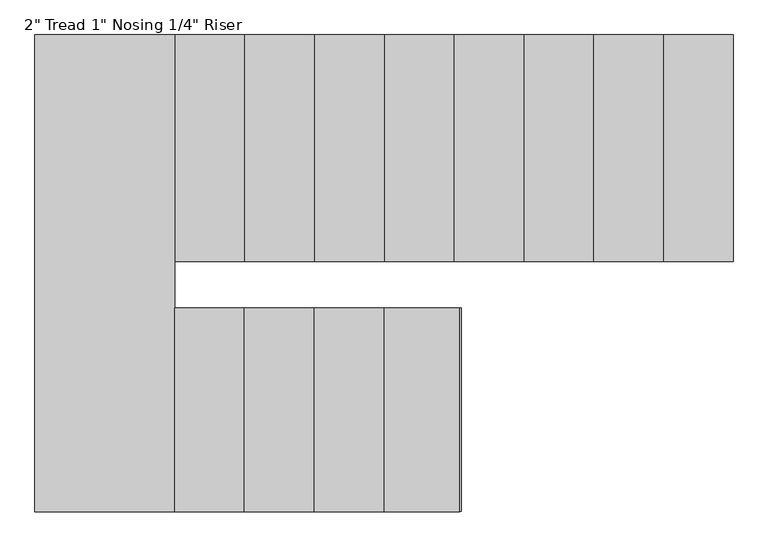
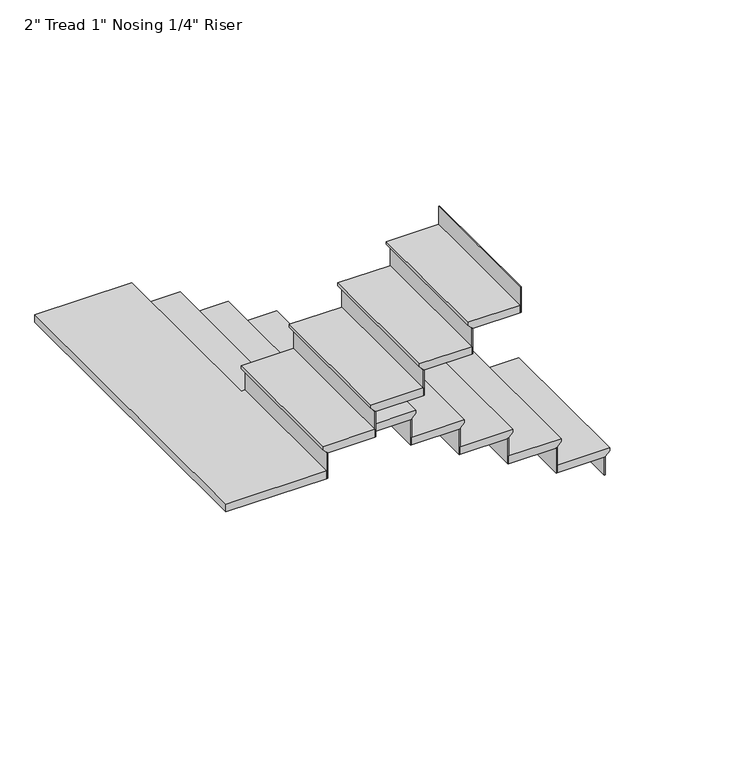
"""IFC4 building model written with IfcOpenShell, lengths in millimetres: stair flight geometry."""

from ifc_helpers import new_model, si_unit, origin, place, context, project, spatial, faceted_brep, source, transform, mapped, element, save


def stair_flight_d10e185a(model_context):
    return source(origin(), model_context, "Body", "Brep", [
        faceted_brep([(-569.5630704, 657.3457979, 3198.2833333), (-569.5630704, 657.3457979, 3217.3333333), (-569.5630704, -333.2542021, 3217.3333333), (-569.5630704, -333.2542021, 3198.2833333), (-594.9630704, 657.3457979, 3172.8833333), (-594.9630704, -333.2542021, 3172.8833333), (-899.7630704, 657.3457979, 3217.3333333), (-899.7630704, -333.2542021, 3217.3333333), (-594.9630704, -333.2542021, 3166.5333333), (-899.7630704, -333.2542021, 3166.5333333), (-899.7630704, 657.3457979, 3166.5333333), (-594.9630704, 657.3457979, 3166.5333333)], [[[0, 1, 2, 3]], [[4, 0, 3, 5]], [[2, 1, 6, 7]], [[8, 9, 10, 11]], [[2, 7, 9, 8, 5, 3]], [[8, 11, 4, 5]], [[6, 1, 0, 4, 11, 10]], [[7, 6, 10, 9]]]),
        faceted_brep([(-594.9630704, 657.3457979, 3166.5333333), (-594.9630704, 657.3457979, 3048.0), (-601.3130704, 657.3457979, 3048.0), (-601.3130704, 657.3457979, 3166.5333333), (-594.9630704, -333.2542021, 3166.5333333), (-601.3130704, -333.2542021, 3166.5333333), (-601.3130704, -333.2542021, 3048.0), (-594.9630704, -333.2542021, 3048.0)], [[[0, 1, 2, 3]], [[4, 5, 6, 7]], [[1, 0, 4, 7]], [[2, 1, 7, 6]], [[3, 2, 6, 5]], [[0, 3, 5, 4]]]),
        faceted_brep([(-899.7630704, 657.3457979, 3335.8666667), (-899.7630704, 657.3457979, 3166.5333333), (-906.1130704, 657.3457979, 3166.5333333), (-906.1130704, 657.3457979, 3335.8666667), (-899.7630704, -333.2542021, 3335.8666667), (-906.1130704, -333.2542021, 3335.8666667), (-906.1130704, -333.2542021, 3166.5333333), (-899.7630704, -333.2542021, 3166.5333333)], [[[0, 1, 2, 3]], [[4, 5, 6, 7]], [[1, 0, 4, 7]], [[2, 1, 7, 6]], [[3, 2, 6, 5]], [[0, 3, 5, 4]]]),
        faceted_brep([(-874.3630704, -333.2542021, 3386.6666667), (-874.3630704, 657.3457979, 3386.6666667), (-1204.5630704, 657.3457979, 3386.6666667), (-1204.5630704, -333.2542021, 3386.6666667), (-899.7630704, -333.2542021, 3335.8666667), (-1204.5630704, -333.2542021, 3335.8666667), (-1204.5630704, 657.3457979, 3335.8666667), (-899.7630704, 657.3457979, 3335.8666667), (-899.7630704, -333.2542021, 3342.2166667), (-874.3630704, -333.2542021, 3367.6166667), (-899.7630704, 657.3457979, 3342.2166667), (-874.3630704, 657.3457979, 3367.6166667)], [[[0, 1, 2, 3]], [[4, 5, 6, 7]], [[0, 3, 5, 4, 8, 9]], [[4, 7, 10, 8]], [[2, 1, 11, 10, 7, 6]], [[3, 2, 6, 5]], [[11, 1, 0, 9]], [[10, 11, 9, 8]]]),
        faceted_brep([(-1204.5630704, 657.3457979, 3505.2), (-1204.5630704, 657.3457979, 3335.8666667), (-1210.9130704, 657.3457979, 3335.8666667), (-1210.9130704, 657.3457979, 3505.2), (-1204.5630704, -333.2542021, 3505.2), (-1210.9130704, -333.2542021, 3505.2), (-1210.9130704, -333.2542021, 3335.8666667), (-1204.5630704, -333.2542021, 3335.8666667)], [[[0, 1, 2, 3]], [[4, 5, 6, 7]], [[1, 0, 4, 7]], [[2, 1, 7, 6]], [[3, 2, 6, 5]], [[0, 3, 5, 4]]]),
        faceted_brep([(-1179.1630704, -333.2542021, 3556.0), (-1179.1630704, 657.3457979, 3556.0), (-1509.3630704, 657.3457979, 3556.0), (-1509.3630704, -333.2542021, 3556.0), (-1204.5630704, -333.2542021, 3505.2), (-1509.3630704, -333.2542021, 3505.2), (-1509.3630704, 657.3457979, 3505.2), (-1204.5630704, 657.3457979, 3505.2), (-1204.5630704, -333.2542021, 3511.55), (-1179.1630704, -333.2542021, 3536.95), (-1204.5630704, 657.3457979, 3511.55), (-1179.1630704, 657.3457979, 3536.95)], [[[0, 1, 2, 3]], [[4, 5, 6, 7]], [[0, 3, 5, 4, 8, 9]], [[4, 7, 10, 8]], [[2, 1, 11, 10, 7, 6]], [[3, 2, 6, 5]], [[11, 1, 0, 9]], [[10, 11, 9, 8]]]),
        faceted_brep([(-1509.3630704, 657.3457979, 3674.5333333), (-1509.3630704, 657.3457979, 3505.2), (-1515.7130704, 657.3457979, 3505.2), (-1515.7130704, 657.3457979, 3674.5333333), (-1509.3630704, -333.2542021, 3674.5333333), (-1515.7130704, -333.2542021, 3674.5333333), (-1515.7130704, -333.2542021, 3505.2), (-1509.3630704, -333.2542021, 3505.2)], [[[0, 1, 2, 3]], [[4, 5, 6, 7]], [[1, 0, 4, 7]], [[2, 1, 7, 6]], [[3, 2, 6, 5]], [[0, 3, 5, 4]]]),
        faceted_brep([(-1483.9630704, -333.2542021, 3725.3333333), (-1483.9630704, 657.3457979, 3725.3333333), (-1814.1630704, 657.3457979, 3725.3333333), (-1814.1630704, -333.2542021, 3725.3333333), (-1509.3630704, -333.2542021, 3674.5333333), (-1814.1630704, -333.2542021, 3674.5333333), (-1814.1630704, 657.3457979, 3674.5333333), (-1509.3630704, 657.3457979, 3674.5333333), (-1509.3630704, -333.2542021, 3680.8833333), (-1483.9630704, -333.2542021, 3706.2833333), (-1509.3630704, 657.3457979, 3680.8833333), (-1483.9630704, 657.3457979, 3706.2833333)], [[[0, 1, 2, 3]], [[4, 5, 6, 7]], [[0, 3, 5, 4, 8, 9]], [[4, 7, 10, 8]], [[2, 1, 11, 10, 7, 6]], [[3, 2, 6, 5]], [[11, 1, 0, 9]], [[10, 11, 9, 8]]]),
        faceted_brep([(-1814.1630704, 657.3457979, 3843.8666667), (-1814.1630704, 657.3457979, 3674.5333333), (-1820.5130704, 657.3457979, 3674.5333333), (-1820.5130704, 657.3457979, 3843.8666667), (-1814.1630704, -333.2542021, 3843.8666667), (-1820.5130704, -333.2542021, 3843.8666667), (-1820.5130704, -333.2542021, 3674.5333333), (-1814.1630704, -333.2542021, 3674.5333333)], [[[0, 1, 2, 3]], [[4, 5, 6, 7]], [[1, 0, 4, 7]], [[2, 1, 7, 6]], [[3, 2, 6, 5]], [[0, 3, 5, 4]]]),
        faceted_brep([(-1788.7630704, -333.2542021, 3894.6666667), (-1788.7630704, 657.3457979, 3894.6666667), (-2118.9630704, 657.3457979, 3894.6666667), (-2118.9630704, -333.2542021, 3894.6666667), (-1814.1630704, -333.2542021, 3843.8666667), (-2118.9630704, -333.2542021, 3843.8666667), (-2118.9630704, 657.3457979, 3843.8666667), (-1814.1630704, 657.3457979, 3843.8666667), (-1814.1630704, -333.2542021, 3850.2166667), (-1788.7630704, -333.2542021, 3875.6166667), (-1814.1630704, 657.3457979, 3850.2166667), (-1788.7630704, 657.3457979, 3875.6166667)], [[[0, 1, 2, 3]], [[4, 5, 6, 7]], [[0, 3, 5, 4, 8, 9]], [[4, 7, 10, 8]], [[2, 1, 11, 10, 7, 6]], [[3, 2, 6, 5]], [[11, 1, 0, 9]], [[10, 11, 9, 8]]]),
        faceted_brep([(-2118.9630704, 657.3457979, 4013.2), (-2118.9630704, 657.3457979, 3843.8666667), (-2125.3130704, 657.3457979, 3843.8666667), (-2125.3130704, 657.3457979, 4013.2), (-2118.9630704, -333.2542021, 4013.2), (-2125.3130704, -333.2542021, 4013.2), (-2125.3130704, -333.2542021, 3843.8666667), (-2118.9630704, -333.2542021, 3843.8666667)], [[[0, 1, 2, 3]], [[4, 5, 6, 7]], [[1, 0, 4, 7]], [[2, 1, 7, 6]], [[3, 2, 6, 5]], [[0, 3, 5, 4]]]),
        faceted_brep([(-2093.5630704, -333.2542021, 4064.0), (-2093.5630704, 657.3457979, 4064.0), (-2423.7630704, 657.3457979, 4064.0), (-2423.7630704, -333.2542021, 4064.0), (-2118.9630704, -333.2542021, 4013.2), (-2423.7630704, -333.2542021, 4013.2), (-2423.7630704, 657.3457979, 4013.2), (-2118.9630704, 657.3457979, 4013.2), (-2118.9630704, -333.2542021, 4019.55), (-2093.5630704, -333.2542021, 4044.95), (-2118.9630704, 657.3457979, 4019.55), (-2093.5630704, 657.3457979, 4044.95)], [[[0, 1, 2, 3]], [[4, 5, 6, 7]], [[0, 3, 5, 4, 8, 9]], [[4, 7, 10, 8]], [[2, 1, 11, 10, 7, 6]], [[3, 2, 6, 5]], [[11, 1, 0, 9]], [[10, 11, 9, 8]]]),
        faceted_brep([(-2423.7630704, 657.3457979, 4182.5333333), (-2423.7630704, 657.3457979, 4013.2), (-2430.1130704, 657.3457979, 4013.2), (-2430.1130704, 657.3457979, 4182.5333333), (-2423.7630704, -333.2542021, 4182.5333333), (-2430.1130704, -333.2542021, 4182.5333333), (-2430.1130704, -333.2542021, 4013.2), (-2423.7630704, -333.2542021, 4013.2)], [[[0, 1, 2, 3]], [[4, 5, 6, 7]], [[1, 0, 4, 7]], [[2, 1, 7, 6]], [[3, 2, 6, 5]], [[0, 3, 5, 4]]]),
        faceted_brep([(-2398.3630704, -333.2542021, 4233.3333333), (-2398.3630704, 657.3457979, 4233.3333333), (-2728.5630704, 657.3457979, 4233.3333333), (-2728.5630704, -333.2542021, 4233.3333333), (-2423.7630704, -333.2542021, 4182.5333333), (-2728.5630704, -333.2542021, 4182.5333333), (-2728.5630704, 657.3457979, 4182.5333333), (-2423.7630704, 657.3457979, 4182.5333333), (-2423.7630704, -333.2542021, 4188.8833333), (-2398.3630704, -333.2542021, 4214.2833333), (-2423.7630704, 657.3457979, 4188.8833333), (-2398.3630704, 657.3457979, 4214.2833333)], [[[0, 1, 2, 3]], [[4, 5, 6, 7]], [[0, 3, 5, 4, 8, 9]], [[4, 7, 10, 8]], [[2, 1, 11, 10, 7, 6]], [[3, 2, 6, 5]], [[11, 1, 0, 9]], [[10, 11, 9, 8]]]),
        faceted_brep([(-2728.5630704, 657.3457979, 4351.8666667), (-2728.5630704, 657.3457979, 4182.5333333), (-2734.9130704, 657.3457979, 4182.5333333), (-2734.9130704, 657.3457979, 4351.8666667), (-2728.5630704, -333.2542021, 4351.8666667), (-2734.9130704, -333.2542021, 4351.8666667), (-2734.9130704, -333.2542021, 4182.5333333), (-2728.5630704, -333.2542021, 4182.5333333)], [[[0, 1, 2, 3]], [[4, 5, 6, 7]], [[1, 0, 4, 7]], [[2, 1, 7, 6]], [[3, 2, 6, 5]], [[0, 3, 5, 4]]]),
        faceted_brep([(-2703.1630704, -333.2542021, 4402.6666667), (-2703.1630704, 657.3457979, 4402.6666667), (-3033.3630704, 657.3457979, 4402.6666667), (-3033.3630704, -333.2542021, 4402.6666667), (-2728.5630704, -333.2542021, 4351.8666667), (-3033.3630704, -333.2542021, 4351.8666667), (-3033.3630704, 657.3457979, 4351.8666667), (-2728.5630704, 657.3457979, 4351.8666667), (-2728.5630704, -333.2542021, 4358.2166667), (-2703.1630704, -333.2542021, 4383.6166667), (-2728.5630704, 657.3457979, 4358.2166667), (-2703.1630704, 657.3457979, 4383.6166667)], [[[0, 1, 2, 3]], [[4, 5, 6, 7]], [[0, 3, 5, 4, 8, 9]], [[4, 7, 10, 8]], [[2, 1, 11, 10, 7, 6]], [[3, 2, 6, 5]], [[11, 1, 0, 9]], [[10, 11, 9, 8]]]),
        faceted_brep([(-3033.3630704, 657.3457979, 4521.2), (-3033.3630704, 657.3457979, 4351.8666667), (-3039.7130704, 657.3457979, 4351.8666667), (-3039.7130704, 657.3457979, 4521.2), (-3033.3630704, -333.2542021, 4521.2), (-3039.7130704, -333.2542021, 4521.2), (-3039.7130704, -333.2542021, 4351.8666667), (-3033.3630704, -333.2542021, 4351.8666667)], [[[0, 1, 2, 3]], [[4, 5, 6, 7]], [[1, 0, 4, 7]], [[2, 1, 7, 6]], [[3, 2, 6, 5]], [[0, 3, 5, 4]]]),
        faceted_brep([(-2982.5630704, -536.4542021, 4572.0), (-3007.9630704, -536.4542021, 4572.0), (-3007.9630704, 657.3457979, 4572.0), (-3617.5630704, 657.3457979, 4572.0), (-3617.5630704, -1425.4542021, 4572.0), (-2982.5630704, -1425.4542021, 4572.0), (-3007.9630704, -536.4542021, 4521.2), (-2982.5630704, -536.4542021, 4521.2), (-2982.5630704, -1425.4542021, 4521.2), (-3617.5630704, -1425.4542021, 4521.2), (-3617.5630704, 657.3457979, 4521.2), (-3033.3630704, 657.3457979, 4521.2), (-3033.3630704, -333.2542021, 4521.2), (-3007.9630704, -333.2542021, 4521.2), (-3007.9630704, -333.2542021, 4552.95), (-3007.9630704, 657.3457979, 4552.95), (-3033.3630704, -333.2542021, 4527.55), (-3033.3630704, 657.3457979, 4527.55)], [[[0, 1, 2, 3, 4, 5]], [[6, 7, 8, 9, 10, 11, 12, 13]], [[1, 0, 7, 6]], [[2, 1, 6, 13, 14, 15]], [[13, 12, 16, 14]], [[12, 11, 17, 16]], [[3, 2, 15, 17, 11, 10]], [[4, 3, 10, 9]], [[5, 4, 9, 8]], [[0, 5, 8, 7]], [[17, 15, 14, 16]]]),
        faceted_brep([(-2982.5630704, -1425.4542021, 4690.5333333), (-2982.5630704, -1425.4542021, 4521.2), (-2976.2130704, -1425.4542021, 4521.2), (-2976.2130704, -1425.4542021, 4690.5333333), (-2982.5630704, -536.4542021, 4690.5333333), (-2976.2130704, -536.4542021, 4690.5333333), (-2976.2130704, -536.4542021, 4521.2), (-2982.5630704, -536.4542021, 4521.2)], [[[0, 1, 2, 3]], [[4, 5, 6, 7]], [[1, 0, 4, 7]], [[2, 1, 7, 6]], [[3, 2, 6, 5]], [[0, 3, 5, 4]]]),
        faceted_brep([(-3007.9630704, -536.4542021, 4741.3333333), (-3007.9630704, -1425.4542021, 4741.3333333), (-2677.7630704, -1425.4542021, 4741.3333333), (-2677.7630704, -536.4542021, 4741.3333333), (-2982.5630704, -536.4542021, 4690.5333333), (-2677.7630704, -536.4542021, 4690.5333333), (-2677.7630704, -1425.4542021, 4690.5333333), (-2982.5630704, -1425.4542021, 4690.5333333), (-2982.5630704, -536.4542021, 4696.8833333), (-3007.9630704, -536.4542021, 4722.2833333), (-2982.5630704, -1425.4542021, 4696.8833333), (-3007.9630704, -1425.4542021, 4722.2833333)], [[[0, 1, 2, 3]], [[4, 5, 6, 7]], [[0, 3, 5, 4, 8, 9]], [[4, 7, 10, 8]], [[2, 1, 11, 10, 7, 6]], [[3, 2, 6, 5]], [[11, 1, 0, 9]], [[10, 11, 9, 8]]]),
        faceted_brep([(-2677.7630704, -1425.4542021, 4859.8666667), (-2677.7630704, -1425.4542021, 4690.5333333), (-2671.4130704, -1425.4542021, 4690.5333333), (-2671.4130704, -1425.4542021, 4859.8666667), (-2677.7630704, -536.4542021, 4859.8666667), (-2671.4130704, -536.4542021, 4859.8666667), (-2671.4130704, -536.4542021, 4690.5333333), (-2677.7630704, -536.4542021, 4690.5333333)], [[[0, 1, 2, 3]], [[4, 5, 6, 7]], [[1, 0, 4, 7]], [[2, 1, 7, 6]], [[3, 2, 6, 5]], [[0, 3, 5, 4]]]),
        faceted_brep([(-2703.1630704, -536.4542021, 4910.6666667), (-2703.1630704, -1425.4542021, 4910.6666667), (-2372.9630704, -1425.4542021, 4910.6666667), (-2372.9630704, -536.4542021, 4910.6666667), (-2677.7630704, -536.4542021, 4859.8666667), (-2372.9630704, -536.4542021, 4859.8666667), (-2372.9630704, -1425.4542021, 4859.8666667), (-2677.7630704, -1425.4542021, 4859.8666667), (-2677.7630704, -536.4542021, 4866.2166667), (-2703.1630704, -536.4542021, 4891.6166667), (-2677.7630704, -1425.4542021, 4866.2166667), (-2703.1630704, -1425.4542021, 4891.6166667)], [[[0, 1, 2, 3]], [[4, 5, 6, 7]], [[0, 3, 5, 4, 8, 9]], [[4, 7, 10, 8]], [[2, 1, 11, 10, 7, 6]], [[3, 2, 6, 5]], [[11, 1, 0, 9]], [[10, 11, 9, 8]]]),
        faceted_brep([(-2372.9630704, -1425.4542021, 5029.2), (-2372.9630704, -1425.4542021, 4859.8666667), (-2366.6130704, -1425.4542021, 4859.8666667), (-2366.6130704, -1425.4542021, 5029.2), (-2372.9630704, -536.4542021, 5029.2), (-2366.6130704, -536.4542021, 5029.2), (-2366.6130704, -536.4542021, 4859.8666667), (-2372.9630704, -536.4542021, 4859.8666667)], [[[0, 1, 2, 3]], [[4, 5, 6, 7]], [[1, 0, 4, 7]], [[2, 1, 7, 6]], [[3, 2, 6, 5]], [[0, 3, 5, 4]]]),
        faceted_brep([(-2398.3630704, -536.4542021, 5080.0), (-2398.3630704, -1425.4542021, 5080.0), (-2068.1630704, -1425.4542021, 5080.0), (-2068.1630704, -536.4542021, 5080.0), (-2372.9630704, -536.4542021, 5029.2), (-2068.1630704, -536.4542021, 5029.2), (-2068.1630704, -1425.4542021, 5029.2), (-2372.9630704, -1425.4542021, 5029.2), (-2372.9630704, -536.4542021, 5035.55), (-2398.3630704, -536.4542021, 5060.95), (-2372.9630704, -1425.4542021, 5035.55), (-2398.3630704, -1425.4542021, 5060.95)], [[[0, 1, 2, 3]], [[4, 5, 6, 7]], [[0, 3, 5, 4, 8, 9]], [[4, 7, 10, 8]], [[2, 1, 11, 10, 7, 6]], [[3, 2, 6, 5]], [[11, 1, 0, 9]], [[10, 11, 9, 8]]]),
        faceted_brep([(-2068.1630704, -1425.4542021, 5198.5333333), (-2068.1630704, -1425.4542021, 5029.2), (-2061.8130704, -1425.4542021, 5029.2), (-2061.8130704, -1425.4542021, 5198.5333333), (-2068.1630704, -536.4542021, 5198.5333333), (-2061.8130704, -536.4542021, 5198.5333333), (-2061.8130704, -536.4542021, 5029.2), (-2068.1630704, -536.4542021, 5029.2)], [[[0, 1, 2, 3]], [[4, 5, 6, 7]], [[1, 0, 4, 7]], [[2, 1, 7, 6]], [[3, 2, 6, 5]], [[0, 3, 5, 4]]]),
        faceted_brep([(-1763.3630704, -1425.4542021, 5367.8666667), (-1763.3630704, -1425.4542021, 5198.5333333), (-1757.0130704, -1425.4542021, 5198.5333333), (-1757.0130704, -1425.4542021, 5367.8666667), (-1763.3630704, -536.4542021, 5367.8666667), (-1757.0130704, -536.4542021, 5367.8666667), (-1757.0130704, -536.4542021, 5198.5333333), (-1763.3630704, -536.4542021, 5198.5333333)], [[[0, 1, 2, 3]], [[4, 5, 6, 7]], [[1, 0, 4, 7]], [[2, 1, 7, 6]], [[3, 2, 6, 5]], [[0, 3, 5, 4]]]),
        faceted_brep([(-2093.5630704, -536.4542021, 5249.3333333), (-2093.5630704, -1425.4542021, 5249.3333333), (-1763.3630704, -1425.4542021, 5249.3333333), (-1763.3630704, -536.4542021, 5249.3333333), (-2068.1630704, -536.4542021, 5198.5333333), (-1763.3630704, -536.4542021, 5198.5333333), (-1763.3630704, -1425.4542021, 5198.5333333), (-2068.1630704, -1425.4542021, 5198.5333333), (-2068.1630704, -536.4542021, 5204.8833333), (-2093.5630704, -536.4542021, 5230.2833333), (-2068.1630704, -1425.4542021, 5204.8833333), (-2093.5630704, -1425.4542021, 5230.2833333)], [[[0, 1, 2, 3]], [[4, 5, 6, 7]], [[0, 3, 5, 4, 8, 9]], [[4, 7, 10, 8]], [[2, 1, 11, 10, 7, 6]], [[3, 2, 6, 5]], [[11, 1, 0, 9]], [[10, 11, 9, 8]]]),
    ])


if __name__ == "__main__":
    model = new_model("IFC4")
    model_context = context("Model", 3, world=origin())
    ifc_project = project(units=[si_unit("LENGTHUNIT", "METRE", prefix="MILLI")], contexts=[model_context])
    site = spatial("IfcSite", under=ifc_project)
    building = spatial("IfcBuilding", under=site)
    placement = place(None, origin())
    stair_flight_shape = stair_flight_d10e185a(model_context)
    element("IfcStairFlight", 1, ObjectType="2\" Tread 1\" Nosing 1/4\" Riser", at=placement, inside=building, context=model_context, shape_type="MappedRepresentation", body=[
        mapped(stair_flight_shape, transform((0.0, 0.0, 0.0), x_axis=(1.0, 0.0, 0.0), y_axis=(0.0, 1.0, 0.0), z_axis=(0.0, 0.0, 1.0))),
    ])
    save(model, "model.ifc")
